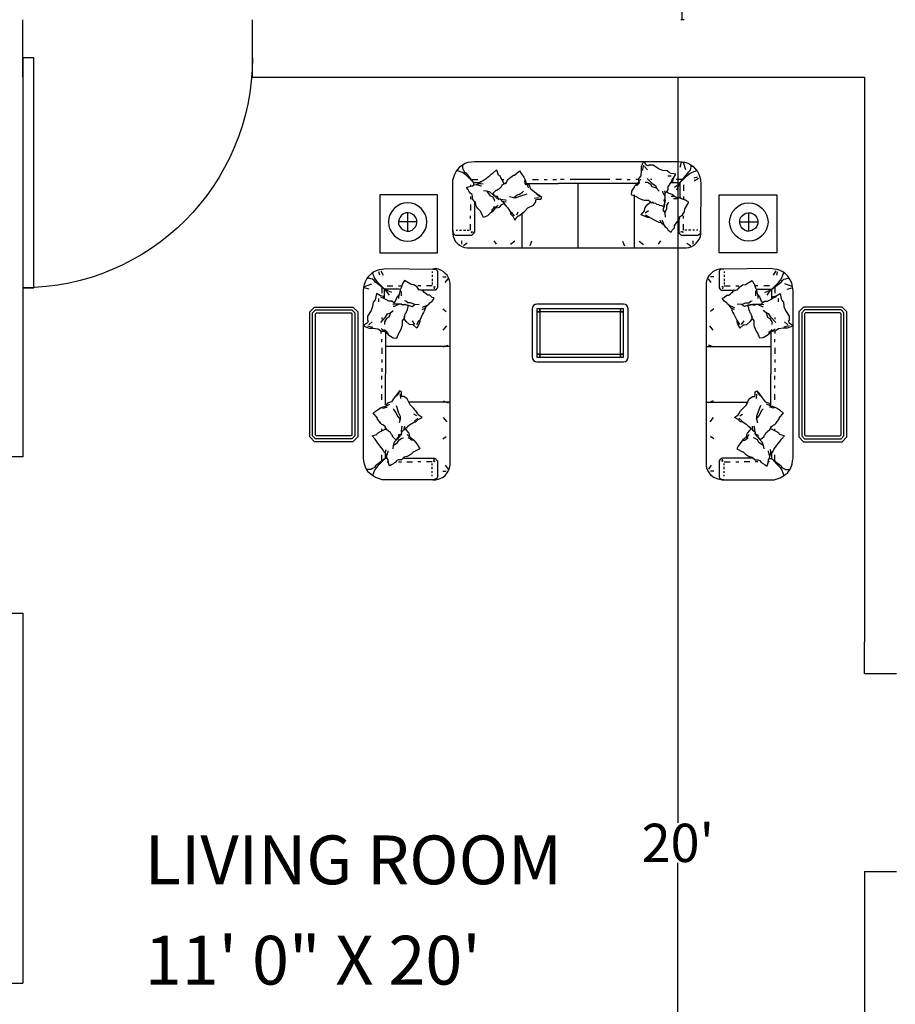
# Model space of a CAD drawing. Units: inches. Extents: x -113 to 5399, y -1393 to 3302.
# Tile 13 of 40: x 1759 to 1896, y 271 to 426. Entities that reach past the tile are written whole.
import ezdxf

# ---------------------------------------------------------------- set-up
doc = ezdxf.new("R2010")
doc.units = ezdxf.units.IN
doc.header["$MEASUREMENT"] = 0
doc.layers.add('24', color=7, linetype='Continuous')
for name, color, linetype, lineweight in [('A-ANNO-DIMS', 254, 'Continuous', 18), ('A-AREA-IDEN', 4, 'Continuous', 18), ('doors', 2, 'Continuous', 25), ('furniture', 131, 'Continuous', 18), ('walls', 1, 'Continuous', 25)]:
    doc.layers.add(name, color=color, linetype=linetype, lineweight=lineweight)
doc.styles.get("Standard").update_dxf_attribs({"font": 'arial.ttf'})
doc.dimstyles.get("Standard").update_dxf_attribs({"dimtxt": 6, "dimasz": 0.18, "dimexe": 0.18, "dimexo": 0.0625, "dimgap": 0.09, "dimtad": 0, "dimtih": 1, "dimtoh": 1, "dimdec": 1, "dimzin": 0, "dimdsep": 46, "dimlunit": 4, "dimtxsty": 'Standard', "dimblk": 'ARCHTICK', "dimcen": 0.09, "dimadec": 0, "dimazin": 0, "dimtfac": 1, "dimtdec": 1, "dimtofl": 0, "dimtmove": 0, "dimatfit": 3, "dimfxl": 1, "dimtolj": 1, "dimtzin": 0, "dimarcsym": 0})

# ---------------------------------------------------------------- blocks, each defined once
blk = doc.blocks.new('*U3')
for p, q in [((0, 0), (0, -6)), ((36, 0), (36, -6))]:
    blk.add_line(p, q)
blk.add_lwpolyline([(0, 0), (0, 36), (1.75, 36), (1.75, 0)], close=True)
blk.add_arc((0, 0), 36, 0, 90)
blk = doc.blocks.new('DL13712')
at = {"layer": '24'}
for p, q in [((33, 28.5), (-34, 28.5)), ((33.5, -29.5), (-10, -29.5))]:
    blk.add_line(p, q, dxfattribs=at)
blk = doc.blocks.new('DL13976')
at = {"layer": '24'}
for p, q in [((-18, 7.5), (-16, 11)), ((-16, 11), (-13.5, 14)), ((-13.5, 14), (-10.5, 16.5)), ((-10.5, 16.5), (-7, 18.5)), ((-7, 18.5), (-3.5, 19.5)), ((-3.5, 19.5), (0.5, 20)), ((0.5, 20), (4.5, 19.5)), ((4.5, 19.5), (8, 18.5)), ((8, 18.5), (11.5, 16.5)), ((11.5, 16.5), (14.5, 14)), ((14.5, 14), (17, 11)), ((17, 11), (19, 7.5)), ((-19.5, 0), (-19, 4)), ((-19, -4), (-19.5, 0)), ((-19, 4), (-18, 7.5)), ((-9, 2), (-8, 4.5)), ((-9, -0.5), (-9, 2)), ((-9, 0), (10, 0)), ((-8, 4.5), (-6.5, 6.5)), ((-6.5, 6.5), (-4.5, 8)), ((-5.5, 0), (6.5, 0)), ((-4.5, 8), (-2.5, 9)), ((-2.5, 9), (0, 9.5)), ((0, 9.5), (2.5, 9.5)), ((0.5, -9.5), (0.5, 9.5)), ((0.5, -6), (0.5, 6)), ((2.5, 9.5), (5, 8.5)), ((5, 8.5), (7, 7)), ((7, 7), (8.5, 5)), ((8.5, 5), (9.5, 3)), ((9.5, 3), (10, 0.5)), ((10, 0.5), (10, -2)), ((19, 7.5), (20, 4)), ((20, 4), (20.5, 0)), ((20.5, 0), (20, -4)), ((-18, -7.5), (-19, -4)), ((-16, -11), (-18, -7.5)), ((-8.5, -3), (-9, -0.5)), ((-7.5, -5), (-8.5, -3)), ((-6, -7), (-7.5, -5)), ((-4, -8.5), (-6, -7)), ((-1.5, -9.5), (-4, -8.5)), ((1, -9.5), (-1.5, -9.5)), ((3.5, -9), (1, -9.5)), ((5.5, -8), (3.5, -9)), ((7.5, -6.5), (5.5, -8)), ((9, -4.5), (7.5, -6.5)), ((10, -2), (9, -4.5)), ((19, -7.5), (17, -11)), ((20, -4), (19, -7.5)), ((-13.5, -14), (-16, -11)), ((-10.5, -16.5), (-13.5, -14)), ((-7, -18.5), (-10.5, -16.5)), ((-3.5, -19.5), (-7, -18.5)), ((0.5, -20), (-3.5, -19.5)), ((4.5, -19.5), (0.5, -20)), ((8, -18.5), (4.5, -19.5)), ((11.5, -16.5), (8, -18.5)), ((14.5, -14), (11.5, -16.5)), ((17, -11), (14.5, -14))]:
    blk.add_line(p, q, dxfattribs=at)
blk = doc.blocks.new('DL13329')
at = {"layer": '24'}
for p, q in [((0, 0), (0, -60)), ((60, 0), (0, 0)), ((60, -60), (60, 0)), ((0, -60), (60, -60))]:
    blk.add_line(p, q, dxfattribs=at)
blk = doc.blocks.new('DL13303')
at = {"layer": '24'}
for p, q in [((-70, 20), (-65, 25)), ((-67, 19), (-64, 22)), ((-65, 25), (65, 25)), ((-64, 22), (64, 22)), ((64, 22), (67, 19)), ((65, 25), (70, 20)), ((-70, -20), (-70, 20)), ((-67, -19), (-67, 19)), ((-64, 18), (-63, 19)), ((-64, -18), (-64, 18)), ((-63, 19), (63, 19)), ((63, 19), (64, 18)), ((64, 18), (64, -18)), ((67, 19), (67, -19)), ((70, 20), (70, -20)), ((-65, -25), (-70, -20)), ((-64, -22), (-67, -19)), ((-63, -19), (-64, -18)), ((63, -19), (-63, -19)), ((64, -18), (63, -19)), ((67, -19), (64, -22)), ((70, -20), (65, -25)), ((65, -25), (-65, -25)), ((64, -22), (-64, -22))]:
    blk.add_line(p, q, dxfattribs=at)
blk = doc.blocks.new('DL12701')
at = {"layer": '24'}
for p, q in [((-102, 40), (-99.5, 42)), ((-99.5, 42), (-96.5, 43.5)), ((-99, 40), (-99, 42)), ((-96.5, 43.5), (-93.5, 44.5)), ((-93.5, 44.5), (-90, 45)), ((-90, 45), (-87, 45.5)), ((-87, 45.5), (0, 45.5)), ((0, 45.5), (87, 45.5)), ((50, 45), (48, 39.5)), ((50.5, 41.5), (49, 36)), ((51.5, 44.5), (50, 45)), ((53.5, 41.5), (51.5, 44.5)), ((55.5, 40.5), (53.5, 41.5)), ((56, 41.5), (55.5, 40.5)), ((60.5, 41.5), (56, 41.5)), ((66.5, 37.5), (60.5, 41.5)), ((87, 45.5), (90.5, 45)), ((88.5, 39.5), (90, 44.5)), ((90.5, 45), (93.5, 44.5)), ((91.5, 44.5), (94, 37)), ((93.5, 44.5), (96.5, 43.5)), ((96.5, 43.5), (99.5, 42)), ((99.5, 42), (102, 40)), ((100, 40), (99.5, 42)), ((-108.5, 29), (-107.5, 32)), ((-107.5, 32), (-106, 35)), ((-106, 35), (-104, 37.5)), ((-102.5, 35), (-105, 36)), ((-104, 37.5), (-102, 40)), ((-99.5, 34), (-102.5, 35)), ((-97, 32), (-99.5, 34)), ((-99, 38), (-99, 40)), ((-98, 36), (-99, 38)), ((-97, 34), (-98, 36)), ((-95, 33), (-97, 34)), ((-95, 30.5), (-97, 32)), ((-87.5, 23), (-95, 33)), ((-71.5, 30.5), (-69.5, 32)), ((-69.5, 32), (-67.5, 33.5)), ((-67.5, 33.5), (-64, 36.5)), ((-64, 36.5), (-62.5, 31.5)), ((-62.5, 31.5), (-61, 31)), ((-61, 31), (-59.5, 28)), ((-49, 29), (-46.5, 31)), ((-46.5, 31), (-45.5, 31)), ((-45.5, 31), (-40, 35.5)), ((-40, 35.5), (-38.5, 33)), ((-38.5, 33), (-38, 32.5)), ((-38, 32.5), (-35.5, 29)), ((48, 35.5), (47.5, 30.5)), ((48, 39.5), (48, 35.5)), ((51.5, 40), (54.5, 36.5)), ((70.5, 36), (66.5, 37.5)), ((75, 35.5), (70.5, 36)), ((77.5, 33.5), (75, 35.5)), ((79, 33), (77.5, 33.5)), ((84, 32), (79, 33)), ((81.5, 28), (84, 32)), ((88.5, 23.5), (96, 33)), ((95.5, 30.5), (98, 32.5)), ((96, 33), (97.5, 34.5)), ((97.5, 34.5), (99, 36)), ((98, 32.5), (100.5, 34)), ((99, 36), (99.5, 38)), ((99.5, 38), (100, 40)), ((100.5, 34), (103, 35)), ((102, 40), (104.5, 37.5)), ((103, 35), (106, 36)), ((104.5, 37.5), (106.5, 35)), ((106.5, 35), (108, 32)), ((108, 32), (109, 29)), ((-109.5, 26), (-108.5, 29)), ((-109.5, 22.5), (-109.5, 26)), ((-109.5, -26.5), (-109.5, 22.5)), ((-87.5, 23), (-95, 30.5)), ((-91, 21), (-91, 19.5)), ((-89.5, 26.5), (-83.5, 26.5)), ((-89, 20), (-87.5, 21)), ((-87.5, 21), (-87.5, 23)), ((-81.5, 23), (-87.5, 23)), ((-87.5, 21), (-85, 21.5)), ((-85, 21.5), (-82, 22.5)), ((-85, 21.5), (-80.5, 20)), ((-82, 22.5), (-80.5, 24.5)), ((-82, 22.5), (-80.5, 22.5)), ((-80.5, 24.5), (-78, 25.5)), ((-80.5, 24.5), (-80.5, 23.5)), ((-80.5, 22.5), (-78, 22)), ((-78, 25.5), (-76, 27)), ((-77, 25.5), (-77, 25.5)), ((-76, 27), (-71.5, 30.5)), ((-59.5, 28), (-57.5, 24.5)), ((-58.5, 19.5), (-58, 21)), ((-58, 26.5), (-56.5, 26.5)), ((-58, 21), (-54.5, 23)), ((-57.5, 24.5), (-56.5, 22)), ((-56.5, 22.5), (-54.5, 22.5)), ((-54.5, 22.5), (-52.5, 25.5)), ((-54.5, 23), (-54.5, 22.5)), ((-54, 22.5), (-54, 22.5)), ((-52.5, 25.5), (-52, 26.5)), ((-52, 26.5), (-51, 27.5)), ((-51, 27.5), (-49, 29)), ((-35.5, 29), (-34.5, 27)), ((-34.5, 27), (-35, 24.5)), ((-35, 24.5), (-34.5, 23)), ((-34.5, 27), (-33.5, 24)), ((-34.5, 23), (-34, 21)), ((-33.5, 24), (-33, 22)), ((-30, 21), (-33, 22)), ((-33, 22), (-31.5, 19.5)), ((-32, 22.5), (0.5, 22.5)), ((-29.5, 19.5), (-30, 21)), ((-26.5, 26.5), (-20.5, 26.5)), ((-14.5, 26.5), (-11.5, 26.5)), ((-5.5, 26.5), (-1.5, 26.5)), ((44, 22.5), (0.5, 22.5)), ((6.5, 26.5), (2.5, 26.5)), ((15.5, 26.5), (12.5, 26.5)), ((27.5, 26.5), (21.5, 26.5)), ((33.5, 26.5), (36.5, 26.5)), ((43.5, 22), (41.5, 20)), ((43.5, 20.5), (41.5, 20)), ((42.5, 27), (45, 27)), ((45, 23.5), (43.5, 22)), ((45, 22), (43.5, 20.5)), ((45.5, 28), (45, 27)), ((45, 27), (45, 23.5)), ((45, 23.5), (46.5, 26)), ((46.5, 23.5), (45, 22)), ((47.5, 30.5), (45.5, 28)), ((46.5, 26), (47.5, 27)), ((54.5, 23.5), (52, 23.5)), ((54, 27.5), (59.5, 22.5)), ((58, 21.5), (54.5, 23.5)), ((59, 26.5), (57.5, 26.5)), ((59.5, 19), (58, 21.5)), ((59.5, 22.5), (63, 20.5)), ((63, 20.5), (64, 17.5)), ((79, 30), (75.5, 30)), ((76, 19), (79, 24)), ((80.5, 28), (79, 24)), ((79, 24), (81, 24.5)), ((79, 23.5), (88.5, 23.5)), ((81, 24.5), (81.5, 28)), ((82.5, 18.5), (88, 22.5)), ((90.5, 26.5), (84.5, 26.5)), ((85, 16), (88, 22.5)), ((88.5, 23.5), (95.5, 30.5)), ((88.5, 8), (88.5, 23.5)), ((92, 21), (92, 15)), ((103, 28.5), (106.5, 29.5)), ((107.5, 27.5), (103, 25)), ((109, 29), (109.5, 26)), ((109.5, 26), (110, 22.5)), ((110, 22.5), (109.5, -26.5)), ((-95, 18.5), (-92, 19.5)), ((-95, 18), (-95, 18.5)), ((-94, 16.5), (-95, 18)), ((-92.5, 14), (-94, 16.5)), ((-92, 13.5), (-92.5, 14)), ((-92, 19.5), (-89, 20)), ((-91.5, 12.5), (-92, 13.5)), ((-89.5, 11), (-91.5, 12.5)), ((-89, 9), (-89.5, 11)), ((-80.5, 20), (-79.5, 20)), ((-74, 14.5), (-77.5, 15)), ((-70.5, 13.5), (-74, 14.5)), ((-74, 14.5), (-71, 10)), ((-67.5, 10.5), (-70.5, 13.5)), ((-68, 12), (-67.5, 12.5)), ((-65, 9), (-68, 12)), ((-67.5, 12.5), (-66.5, 13.5)), ((-61.5, 5.5), (-67.5, 10.5)), ((-66.5, 13.5), (-64.5, 15.5)), ((-64.5, 15.5), (-63.5, 15.5)), ((-63.5, 15.5), (-62.5, 16.5)), ((-62.5, 16.5), (-60.5, 17.5)), ((-60.5, 17.5), (-59, 19.5)), ((-59, 19.5), (-58.5, 19.5)), ((-46.5, 7.5), (-42.5, 10.5)), ((-42.5, 10.5), (-40, 11.5)), ((-40, 11.5), (-37, 13.5)), ((-32.5, 11.5), (-40, 9)), ((-37, 13.5), (-36, 14.5)), ((-31.5, 19.5), (-31, 18)), ((-28.5, 16.5), (-29.5, 19.5)), ((-24.5, 13.5), (-28.5, 16.5)), ((-21, 11), (-24.5, 13.5)), ((-19, 8.5), (-22.5, 11.5)), ((-17, 8), (-21, 11)), ((38, 14), (37.5, 11)), ((37.5, 11), (43.5, 8.5)), ((40.5, 18.5), (38, 14.5)), ((38, 14.5), (38, 14)), ((41.5, 20), (40.5, 18.5)), ((64, 17.5), (59.5, 19)), ((64, 17.5), (66.5, 14.5)), ((70.5, 13.5), (70.5, 14.5)), ((73, 8.5), (70.5, 13.5)), ((73, 13), (72.5, 15)), ((73, 12.5), (75, 14.5)), ((73, 12.5), (73, 13)), ((73, 8.5), (73, 12.5)), ((76, 12.5), (74, 14)), ((75, 14.5), (76, 16)), ((75.5, 16), (76, 16.5)), ((76, 16), (76, 19)), ((80, 11), (76, 12.5)), ((80.5, 10.5), (80, 11)), ((83, 8.5), (80.5, 10.5)), ((-91, 9), (-91, 6)), ((-91, 0.5), (-91, -5.5)), ((-89, 8.5), (-89, 9)), ((-89, 6), (-89, 8.5)), ((-86.5, 3.5), (-89, 6)), ((-87, 3.5), (-87, -26.5)), ((-86, 3.5), (-86.5, 3.5)), ((-85.5, 0.5), (-86, 3.5)), ((-85.5, 0), (-85.5, 0.5)), ((-84.5, -2), (-85.5, 0)), ((-71, 10), (-68, 8.5)), ((-68, 8.5), (-66.5, 5.5)), ((-66.5, 5.5), (-66, 4)), ((-63, 9), (-65, 9)), ((-62.5, 0), (-63.5, -1)), ((-62, 6.5), (-63, 9)), ((-60, 6), (-62, 6.5)), ((-61, -2), (-58.5, 0.5)), ((-57.5, 3.5), (-60, 6)), ((-60, 6), (-55, 5.5)), ((-58.5, 0.5), (-55.5, 2)), ((-56.5, 3.5), (-57.5, 3.5)), ((-57.5, 3.5), (-56, 1.5)), ((-54, 3), (-56.5, 3.5)), ((-56, 1.5), (-55, 0)), ((-55, 5.5), (-54, 5)), ((-55, 0), (-52.5, -2.5)), ((-46.5, 7.5), (-50.5, 8.5)), ((-43.5, 7.5), (-46.5, 7.5)), ((-40, 9), (-43.5, 7.5)), ((-31.5, -3), (-25.5, 0)), ((-25.5, 0), (-23, 3.5)), ((-20.5, 7.5), (-25, 7)), ((-23, 5.5), (-21.5, 6)), ((-23, 3.5), (-23, 5.5)), ((-21.5, 6), (-18, 6)), ((-18, 6), (-17, 8)), ((43.5, 8.5), (44, 8)), ((44, 8), (47, 6.5)), ((47, 6.5), (49.5, 5.5)), ((49.5, 5.5), (51, 5)), ((51, 5), (52.5, 5)), ((52, -2.5), (55, 1)), ((52.5, 5), (55.5, 5)), ((55, 1), (57.5, 3)), ((55.5, 5), (55.5, 5)), ((55.5, 5), (59, 2.5)), ((59, 2.5), (60, 3.5)), ((60, 3.5), (60, 2.5)), ((60, 2.5), (63, 2)), ((63, 2), (64, 1)), ((64, 1), (66, 0.5)), ((66, 0.5), (66.5, 0)), ((66.5, 0), (69, -0.5)), ((71.5, -1), (72.5, 2.5)), ((72, 5), (73, 6.5)), ((73, 5.5), (72, -1)), ((72.5, 2.5), (72, 5)), ((73, 6.5), (73, 8.5)), ((74.5, -0.5), (76, 1.5)), ((76, 1.5), (76.5, 3)), ((80.5, 9), (79, 9)), ((83, 8.5), (80.5, 9)), ((84, 6.5), (81.5, 6.5)), ((85, 8), (83, 8.5)), ((85.5, 6.5), (84, 6.5)), ((88, 7.5), (85, 8)), ((88, 7.5), (85.5, 6.5)), ((90, 6.5), (88, 7.5)), ((94, 5), (90, 6.5)), ((92, 9), (92, 6)), ((95, 4.5), (94, 5)), ((94, -3), (97.5, 3)), ((97.5, 3), (95, 4.5)), ((-83, -4), (-84.5, -2)), ((-80.5, -6.5), (-83, -4)), ((-80.5, -7), (-80.5, -6.5)), ((-77.5, -13), (-80.5, -7)), ((-70.5, -8.5), (-73.5, -11)), ((-68.5, -7), (-70.5, -8.5)), ((-68.5, -4.5), (-67, -3)), ((-66.5, -4.5), (-68.5, -7)), ((-68.5, -7), (-68.5, -4.5)), ((-67, -3), (-66, -1)), ((-65.5, -3), (-66.5, -4.5)), ((-63.5, -1), (-65.5, -3)), ((-65.5, -3), (-62.5, -2.5)), ((-62.5, -2.5), (-61, -2)), ((-54, -0.5), (-53.5, -0.5)), ((-52.5, -2.5), (-49.5, -7.5)), ((-49.5, -7.5), (-49.5, -9)), ((-49.5, -9), (-47, -11.5)), ((-45.5, -11), (-48.5, -7.5)), ((-43, -10), (-41.5, -7)), ((-41, -11), (-38, -9)), ((-38, -9), (-35, -6.5)), ((-35, -6.5), (-31.5, -3)), ((48, -10), (51.5, -6)), ((52, -12), (48, -10)), ((51.5, -5.5), (52, -2.5)), ((51.5, -6), (51.5, -5.5)), ((52, -8), (55.5, -5.5)), ((52, -10), (56.5, -12.5)), ((69, -0.5), (70.5, -1)), ((70.5, -1), (71.5, -1)), ((72, -1), (70.5, -5)), ((70.5, -5), (72.5, -8)), ((72.5, -8), (74.5, -3.5)), ((72.5, -8), (73, -12.5)), ((74.5, -3.5), (74.5, -0.5)), ((89.5, -11), (91, -10)), ((91, -10), (92, -8.5)), ((92, -8.5), (93, -7)), ((93, -7), (93.5, -4)), ((93.5, -4), (94, -3)), ((-91, -14), (-91, -11)), ((-91, -26), (-91, -20)), ((-74.5, -11.5), (-77.5, -13)), ((-73.5, -11), (-74.5, -11.5)), ((-47, -11.5), (-45, -15.5)), ((-45, -15.5), (-42, -11.5)), ((-42, -11.5), (-41, -11)), ((55, -13), (52, -12)), ((56.5, -13), (55, -13)), ((62.5, -16), (56.5, -13)), ((64.5, -17), (62.5, -16)), ((64, -16.5), (64, -16.5)), ((66.5, -18), (64.5, -17)), ((69, -18.5), (66.5, -18)), ((67.5, -15.5), (68.5, -18)), ((68.5, -18), (69, -18.5)), ((69, -18.5), (72, -21)), ((70, -16.5), (69.5, -15.5)), ((72, -21), (70, -16.5)), ((82.5, -21.5), (83.5, -20)), ((83.5, -20), (85, -18)), ((85, -17.5), (87, -16.5)), ((85, -18), (85, -17.5)), ((87, -16.5), (88, -13)), ((87.5, -12.5), (89.5, -11)), ((88, -13), (87.5, -12.5)), ((87.5, -26.5), (87.5, -14.5)), ((92, -14), (92, -11)), ((92, -26), (92, -20)), ((-109.5, -28), (-109.5, -26.5)), ((-109.5, -26.5), (-109.5, -29.5)), ((-109, -29), (-109.5, -28)), ((-109.5, -29.5), (-109, -32.5)), ((-108.5, -30), (-109, -29)), ((-108, -31), (-108.5, -30)), ((-106, -26), (-104.5, -26)), ((-102.5, -26), (-100.5, -26)), ((-98.5, -26), (-96, -26)), ((-94.5, -26), (-92.5, -26)), ((-90.5, -27.5), (-88, -28)), ((-90.5, -28), (-90, -29)), ((-89, -30.5), (-90, -31.5)), ((-88, -30), (-89, -30.5)), ((-87.5, -29), (-88, -30)), ((-87, -28), (-87.5, -29)), ((-87, -26.5), (-87, -28)), ((72, -21), (73, -22.5)), ((73, -22.5), (74.5, -23.5)), ((74.5, -23.5), (76, -26)), ((76, -26), (79, -28)), ((79, -28), (79.5, -27.5)), ((79.5, -27.5), (80, -26)), ((80, -26), (82.5, -23.5)), ((82.5, -22.5), (82.5, -21.5)), ((82.5, -23.5), (82.5, -22.5)), ((87.5, -28), (87.5, -26.5)), ((87.5, -29), (87.5, -28)), ((88, -30), (87.5, -29)), ((89, -30.5), (88, -30)), ((91.5, -27.5), (89, -28)), ((90, -31.5), (89, -30.5)), ((91.5, -28), (91, -29)), ((95.5, -26), (93.5, -26)), ((99.5, -26), (97, -26)), ((103.5, -26), (101.5, -26)), ((107, -26), (105.5, -26)), ((109, -30), (108, -31)), ((109.5, -29), (109, -30)), ((110, -29.5), (109.5, -26.5)), ((109.5, -26.5), (109.5, -28)), ((109.5, -28), (109.5, -29)), ((109.5, -32.5), (110, -29.5)), ((-109, -32.5), (-108, -35)), ((-106.5, -31.5), (-108, -31)), ((-108, -35), (-107, -37.5)), ((-107, -37.5), (-105, -39.5)), ((-105.5, -31.5), (-106.5, -31.5)), ((-104.5, -31.5), (-105.5, -31.5)), ((-105, -39.5), (-102.5, -41.5)), ((-92, -31.5), (-104.5, -31.5)), ((-100.5, -37), (-100.5, -40.5)), ((-94.5, -39.5), (-98.5, -42.5)), ((-91, -31.5), (-92, -31.5)), ((-90, -31.5), (-91, -31.5)), ((-67, -37), (-64.5, -40.5)), ((-45, -37.5), (-49.5, -41)), ((-27.5, -37.5), (-29.5, -42.5)), ((28.5, -37.5), (30.5, -42.5)), ((46, -37.5), (50.5, -41)), ((68, -37), (65.5, -40.5)), ((91, -31.5), (90, -31.5)), ((92.5, -31.5), (91, -31.5)), ((104.5, -31.5), (92.5, -31.5)), ((95.5, -39.5), (99.5, -42.5)), ((101.5, -37), (101.5, -40.5)), ((103, -41.5), (105, -39.5)), ((106, -31.5), (104.5, -31.5)), ((105, -39.5), (107, -37.5)), ((107, -31.5), (106, -31.5)), ((108, -31), (107, -31.5)), ((107, -37.5), (108.5, -35)), ((108.5, -35), (109.5, -32.5)), ((-102.5, -41.5), (-100, -43)), ((-100, -43), (-97.5, -44)), ((-97.5, -44), (-94.5, -44.5)), ((-94.5, -44.5), (0, -44.5)), ((0, -44.5), (95, -44.5)), ((95, -44.5), (97.5, -44)), ((97.5, -44), (100.5, -43)), ((100.5, -43), (103, -41.5))]:
    blk.add_line(p, q, dxfattribs=at)
blk = doc.blocks.new('DL13707')
at = {"layer": '24'}
for p, q in [((0, -33.5), (0, 33.5)), ((-58.5, -33.5), (-58.5, 21.5)), ((58.5, -33.5), (58.5, 2))]:
    blk.add_line(p, q, dxfattribs=at)
blk = doc.blocks.new('DL13651')
at = {"layer": '24'}
for p, q in [((-50.5, 25), (-50, 27)), ((-50.5, -25), (-50.5, 25)), ((-50, 27), (-49, 28.5)), ((-49, 28.5), (-47.5, 29.5)), ((-47.5, 29.5), (-45.5, 30)), ((-45.5, 30), (44.5, 30)), ((-45.5, 24.5), (-45.5, 25)), ((-45.5, 25), (-45, 25)), ((-45.5, -24.5), (-45.5, 24.5)), ((-45, 25), (44, 25)), ((-45, 22), (44, 22)), ((-42.5, 22), (-45, 22)), ((-42.5, -24.5), (-42.5, 24.5)), ((-42.5, 24.5), (-42.5, 22)), ((41.5, 22), (41.5, 24.5)), ((41.5, 24.5), (41.5, -24.5)), ((44, 22), (41.5, 22)), ((44, 25), (44.5, 25)), ((44.5, 30), (46.5, 29.5)), ((44.5, 25), (44.5, 24.5)), ((44.5, 24.5), (44.5, -24.5)), ((46.5, 29.5), (48, 28.5)), ((48, 28.5), (49, 27)), ((49, 27), (49.5, 25)), ((49.5, 25), (49.5, -25)), ((-50, -27), (-50.5, -25)), ((-49, -28.5), (-50, -27)), ((-47.5, -29.5), (-49, -28.5)), ((-45.5, -30), (-47.5, -29.5)), ((-45.5, -25), (-45.5, -24.5)), ((-45, -25), (-45.5, -25)), ((44.5, -30), (-45.5, -30)), ((44, -22), (-45, -22)), ((-45, -22), (-42.5, -22)), ((44, -25), (-45, -25)), ((-42.5, -22), (-42.5, -24.5)), ((41.5, -24.5), (41.5, -22)), ((41.5, -22), (44, -22)), ((44.5, -25), (44, -25)), ((44.5, -24.5), (44.5, -25)), ((46.5, -29.5), (44.5, -30)), ((48, -28.5), (46.5, -29.5)), ((49, -27), (48, -28.5)), ((49.5, -25), (49, -27))]:
    blk.add_line(p, q, dxfattribs=at)
blk = doc.blocks.new('DL12263')
at = {"layer": '24'}
for p, q in [((-121, 40), (-118.5, 42)), ((-118.5, 42), (-115.5, 43.5)), ((-118, 40), (-118, 42)), ((-115.5, 43.5), (-112.5, 44.5)), ((-112.5, 44.5), (-109, 45)), ((-109, 45), (-106, 45.5)), ((-106, 45.5), (-19, 45.5)), ((-19, 45.5), (106.5, 45.5)), ((69.5, 45), (67.5, 39.5)), ((70, 41.5), (68.5, 36)), ((71, 44.5), (69.5, 45)), ((73, 41.5), (71, 44.5)), ((75, 40.5), (73, 41.5)), ((75.5, 41.5), (75, 40.5)), ((80, 41.5), (75.5, 41.5)), ((86, 37.5), (80, 41.5)), ((106.5, 45.5), (110, 45)), ((108, 39.5), (109.5, 44.5)), ((110, 45), (113, 44.5)), ((111, 44.5), (113.5, 37)), ((113, 44.5), (116, 43.5)), ((116, 43.5), (119, 42)), ((119, 42), (121.5, 40)), ((119.5, 40), (119, 42)), ((-127.5, 29), (-126.5, 32)), ((-126.5, 32), (-125, 35)), ((-125, 35), (-123, 37.5)), ((-121.5, 35), (-124, 36)), ((-123, 37.5), (-121, 40)), ((-118.5, 34), (-121.5, 35)), ((-116, 32), (-118.5, 34)), ((-118, 38), (-118, 40)), ((-117, 36), (-118, 38)), ((-116, 34), (-117, 36)), ((-114, 33), (-116, 34)), ((-114, 30.5), (-116, 32)), ((-106.5, 23), (-114, 33)), ((-90.5, 30.5), (-88.5, 32)), ((-88.5, 32), (-86.5, 33.5)), ((-86.5, 33.5), (-83, 36.5)), ((-83, 36.5), (-81.5, 31.5)), ((-81.5, 31.5), (-80, 31)), ((-80, 31), (-78.5, 28)), ((-68, 29), (-65.5, 31)), ((-65.5, 31), (-64.5, 31)), ((-64.5, 31), (-59, 35.5)), ((-59, 35.5), (-57.5, 33)), ((-57.5, 33), (-57, 32.5)), ((-57, 32.5), (-54.5, 29)), ((67.5, 35.5), (67, 30.5)), ((67.5, 39.5), (67.5, 35.5)), ((71, 40), (74, 36.5)), ((90, 36), (86, 37.5)), ((94.5, 35.5), (90, 36)), ((97, 33.5), (94.5, 35.5)), ((98.5, 33), (97, 33.5)), ((103.5, 32), (98.5, 33)), ((101, 28), (103.5, 32)), ((108, 23.5), (115.5, 33)), ((115, 30.5), (117.5, 32.5)), ((115.5, 33), (117, 34.5)), ((117, 34.5), (118.5, 36)), ((117.5, 32.5), (120, 34)), ((118.5, 36), (119, 38)), ((119, 38), (119.5, 40)), ((120, 34), (122.5, 35)), ((121.5, 40), (124, 37.5)), ((122.5, 35), (125.5, 36)), ((124, 37.5), (126, 35)), ((126, 35), (127.5, 32)), ((127.5, 32), (128.5, 29)), ((-128.5, 26), (-127.5, 29)), ((-128.5, 22.5), (-128.5, 26)), ((-128.5, -26.5), (-128.5, 22.5)), ((-106.5, 23), (-114, 30.5)), ((-110, 21), (-110, 19.5)), ((-108.5, 26.5), (-102.5, 26.5)), ((-108, 20), (-106.5, 21)), ((-106.5, 21), (-106.5, 23)), ((-100.5, 23), (-106.5, 23)), ((-106.5, 21), (-104, 21.5)), ((-104, 21.5), (-101, 22.5)), ((-104, 21.5), (-99.5, 20)), ((-101, 22.5), (-99.5, 24.5)), ((-101, 22.5), (-99.5, 22.5)), ((-99.5, 24.5), (-97, 25.5)), ((-99.5, 24.5), (-99.5, 23.5)), ((-99.5, 22.5), (-97, 22)), ((-97, 25.5), (-95, 27)), ((-96, 25.5), (-96, 25.5)), ((-95, 27), (-90.5, 30.5)), ((-78.5, 28), (-76.5, 24.5)), ((-77.5, 19.5), (-77, 21)), ((-77, 26.5), (-75.5, 26.5)), ((-77, 21), (-73.5, 23)), ((-76.5, 24.5), (-75.5, 22)), ((-75.5, 22.5), (-73.5, 22.5)), ((-73.5, 22.5), (-71.5, 25.5)), ((-73.5, 23), (-73.5, 22.5)), ((-73, 22.5), (-73, 22.5)), ((-71.5, 25.5), (-71, 26.5)), ((-71, 26.5), (-70, 27.5)), ((-70, 27.5), (-68, 29)), ((-54.5, 29), (-53.5, 27)), ((-53.5, 27), (-54, 24.5)), ((-54, 24.5), (-53.5, 23)), ((-53.5, 27), (-52.5, 24)), ((-53.5, 23), (-53, 21)), ((-52.5, 24), (-52, 22)), ((-49, 21), (-52, 22)), ((-52, 22), (-50.5, 19.5)), ((-51, 22.5), (-18.5, 22.5)), ((-48.5, 19.5), (-49, 21)), ((-45.5, 26.5), (-39.5, 26.5)), ((-33.5, 26.5), (-30.5, 26.5)), ((-24.5, 26.5), (-20.5, 26.5)), ((63.5, 22.5), (-18.5, 22.5)), ((-12.5, 26.5), (-16.5, 26.5)), ((35, 26.5), (-6.5, 26.5)), ((47, 26.5), (41, 26.5)), ((53, 26.5), (56, 26.5)), ((63, 22), (61, 20)), ((63, 20.5), (61, 20)), ((62, 27), (64.5, 27)), ((64.5, 23.5), (63, 22)), ((64.5, 22), (63, 20.5)), ((65, 28), (64.5, 27)), ((64.5, 27), (64.5, 23.5)), ((64.5, 23.5), (66, 26)), ((66, 23.5), (64.5, 22)), ((67, 30.5), (65, 28)), ((66, 26), (67, 27)), ((74, 23.5), (71.5, 23.5)), ((73.5, 27.5), (79, 22.5)), ((77.5, 21.5), (74, 23.5)), ((78.5, 26.5), (77, 26.5)), ((79, 19), (77.5, 21.5)), ((79, 22.5), (82.5, 20.5)), ((82.5, 20.5), (83.5, 17.5)), ((98.5, 30), (95, 30)), ((95.5, 19), (98.5, 24)), ((100, 28), (98.5, 24)), ((98.5, 24), (100.5, 24.5)), ((98.5, 23.5), (108, 23.5)), ((100.5, 24.5), (101, 28)), ((102, 18.5), (107.5, 22.5)), ((110, 26.5), (104, 26.5)), ((104.5, 16), (107.5, 22.5)), ((108, 23.5), (115, 30.5)), ((108, 8), (108, 23.5)), ((111.5, 21), (111.5, 15)), ((122.5, 28.5), (126, 29.5)), ((127, 27.5), (122.5, 25)), ((128.5, 29), (129, 26)), ((129, 26), (129.5, 22.5)), ((129.5, 22.5), (129, -26.5)), ((-114, 18.5), (-111, 19.5)), ((-114, 18), (-114, 18.5)), ((-113, 16.5), (-114, 18)), ((-111.5, 14), (-113, 16.5)), ((-111, 13.5), (-111.5, 14)), ((-111, 19.5), (-108, 20)), ((-110.5, 12.5), (-111, 13.5)), ((-108.5, 11), (-110.5, 12.5)), ((-108, 9), (-108.5, 11)), ((-99.5, 20), (-98.5, 20)), ((-93, 14.5), (-96.5, 15)), ((-89.5, 13.5), (-93, 14.5)), ((-93, 14.5), (-90, 10)), ((-86.5, 10.5), (-89.5, 13.5)), ((-87, 12), (-86.5, 12.5)), ((-84, 9), (-87, 12)), ((-86.5, 12.5), (-85.5, 13.5)), ((-80.5, 5.5), (-86.5, 10.5)), ((-85.5, 13.5), (-83.5, 15.5)), ((-83.5, 15.5), (-82.5, 15.5)), ((-82.5, 15.5), (-81.5, 16.5)), ((-81.5, 16.5), (-79.5, 17.5)), ((-79.5, 17.5), (-78, 19.5)), ((-78, 19.5), (-77.5, 19.5)), ((-65.5, 7.5), (-61.5, 10.5)), ((-61.5, 10.5), (-59, 11.5)), ((-59, 11.5), (-56, 13.5)), ((-51.5, 11.5), (-59, 9)), ((-56, 13.5), (-55, 14.5)), ((-50.5, 19.5), (-50, 18)), ((-47.5, 16.5), (-48.5, 19.5)), ((-43.5, 13.5), (-47.5, 16.5)), ((-40, 11), (-43.5, 13.5)), ((-38, 8.5), (-41.5, 11.5)), ((-36, 8), (-40, 11)), ((57.5, 14), (57, 11)), ((57, 11), (63, 8.5)), ((60, 18.5), (57.5, 14.5)), ((57.5, 14.5), (57.5, 14)), ((61, 20), (60, 18.5)), ((83.5, 17.5), (79, 19)), ((83.5, 17.5), (86, 14.5)), ((90, 13.5), (90, 14.5)), ((92.5, 8.5), (90, 13.5)), ((92.5, 13), (92, 15)), ((92.5, 12.5), (94.5, 14.5)), ((92.5, 12.5), (92.5, 13)), ((92.5, 8.5), (92.5, 12.5)), ((95.5, 12.5), (93.5, 14)), ((94.5, 14.5), (95.5, 16)), ((95, 16), (95.5, 16.5)), ((95.5, 16), (95.5, 19)), ((99.5, 11), (95.5, 12.5)), ((100, 10.5), (99.5, 11)), ((102.5, 8.5), (100, 10.5)), ((-110, 9), (-110, 6)), ((-110, 0.5), (-110, -5.5)), ((-108, 8.5), (-108, 9)), ((-108, 6), (-108, 8.5)), ((-105.5, 3.5), (-108, 6)), ((-106, 3.5), (-106, -26.5)), ((-105, 3.5), (-105.5, 3.5)), ((-104.5, 0.5), (-105, 3.5)), ((-104.5, 0), (-104.5, 0.5)), ((-103.5, -2), (-104.5, 0)), ((-90, 10), (-87, 8.5)), ((-87, 8.5), (-85.5, 5.5)), ((-85.5, 5.5), (-85, 4)), ((-82, 9), (-84, 9)), ((-81.5, 0), (-82.5, -1)), ((-81, 6.5), (-82, 9)), ((-79, 6), (-81, 6.5)), ((-80, -2), (-77.5, 0.5)), ((-76.5, 3.5), (-79, 6)), ((-79, 6), (-74, 5.5)), ((-77.5, 0.5), (-74.5, 2)), ((-75.5, 3.5), (-76.5, 3.5)), ((-76.5, 3.5), (-75, 1.5)), ((-73, 3), (-75.5, 3.5)), ((-75, 1.5), (-74, 0)), ((-74, 5.5), (-73, 5)), ((-74, 0), (-71.5, -2.5)), ((-65.5, 7.5), (-69.5, 8.5)), ((-62.5, 7.5), (-65.5, 7.5)), ((-59, 9), (-62.5, 7.5)), ((-50.5, -3), (-44.5, 0)), ((-44.5, 0), (-42, 3.5)), ((-39.5, 7.5), (-44, 7)), ((-42, 5.5), (-40.5, 6)), ((-42, 3.5), (-42, 5.5)), ((-40.5, 6), (-37, 6)), ((-37, 6), (-36, 8)), ((63, 8.5), (63.5, 8)), ((63.5, 8), (66.5, 6.5)), ((66.5, 6.5), (69, 5.5)), ((69, 5.5), (70.5, 5)), ((70.5, 5), (72, 5)), ((71.5, -2.5), (74.5, 1)), ((72, 5), (75, 5)), ((74.5, 1), (77, 3)), ((75, 5), (75, 5)), ((75, 5), (78.5, 2.5)), ((78.5, 2.5), (79.5, 3.5)), ((79.5, 3.5), (79.5, 2.5)), ((79.5, 2.5), (82.5, 2)), ((82.5, 2), (83.5, 1)), ((83.5, 1), (85.5, 0.5)), ((85.5, 0.5), (86, 0)), ((86, 0), (88.5, -0.5)), ((91, -1), (92, 2.5)), ((91.5, 5), (92.5, 6.5)), ((92.5, 5.5), (91.5, -1)), ((92, 2.5), (91.5, 5)), ((92.5, 6.5), (92.5, 8.5)), ((94, -0.5), (95.5, 1.5)), ((95.5, 1.5), (96, 3)), ((100, 9), (98.5, 9)), ((102.5, 8.5), (100, 9)), ((103.5, 6.5), (101, 6.5)), ((104.5, 8), (102.5, 8.5)), ((105, 6.5), (103.5, 6.5)), ((107.5, 7.5), (104.5, 8)), ((107.5, 7.5), (105, 6.5)), ((109.5, 6.5), (107.5, 7.5)), ((113.5, 5), (109.5, 6.5)), ((111.5, 9), (111.5, 6)), ((114.5, 4.5), (113.5, 5)), ((113.5, -3), (117, 3)), ((117, 3), (114.5, 4.5)), ((-102, -4), (-103.5, -2)), ((-99.5, -6.5), (-102, -4)), ((-99.5, -7), (-99.5, -6.5)), ((-96.5, -13), (-99.5, -7)), ((-89.5, -8.5), (-92.5, -11)), ((-87.5, -7), (-89.5, -8.5)), ((-87.5, -4.5), (-86, -3)), ((-85.5, -4.5), (-87.5, -7)), ((-87.5, -7), (-87.5, -4.5)), ((-86, -3), (-85, -1)), ((-84.5, -3), (-85.5, -4.5)), ((-82.5, -1), (-84.5, -3)), ((-84.5, -3), (-81.5, -2.5)), ((-81.5, -2.5), (-80, -2)), ((-73, -0.5), (-72.5, -0.5)), ((-71.5, -2.5), (-68.5, -7.5)), ((-68.5, -7.5), (-68.5, -9)), ((-68.5, -9), (-66, -11.5)), ((-64.5, -11), (-67.5, -7.5)), ((-62, -10), (-60.5, -7)), ((-60, -11), (-57, -9)), ((-57, -9), (-54, -6.5)), ((-54, -6.5), (-50.5, -3)), ((67.5, -10), (71, -6)), ((71.5, -12), (67.5, -10)), ((71, -5.5), (71.5, -2.5)), ((71, -6), (71, -5.5)), ((71.5, -8), (75, -5.5)), ((71.5, -10), (76, -12.5)), ((88.5, -0.5), (90, -1)), ((90, -1), (91, -1)), ((91.5, -1), (90, -5)), ((90, -5), (92, -8)), ((92, -8), (94, -3.5)), ((92, -8), (92.5, -12.5)), ((94, -3.5), (94, -0.5)), ((109, -11), (110.5, -10)), ((110.5, -10), (111.5, -8.5)), ((111.5, -8.5), (112.5, -7)), ((112.5, -7), (113, -4)), ((113, -4), (113.5, -3)), ((-110, -14), (-110, -11)), ((-110, -26), (-110, -20)), ((-93.5, -11.5), (-96.5, -13)), ((-92.5, -11), (-93.5, -11.5)), ((-66, -11.5), (-64, -15.5)), ((-64, -15.5), (-61, -11.5)), ((-61, -11.5), (-60, -11)), ((74.5, -13), (71.5, -12)), ((76, -13), (74.5, -13)), ((82, -16), (76, -13)), ((84, -17), (82, -16)), ((83.5, -16.5), (83.5, -16.5)), ((86, -18), (84, -17)), ((88.5, -18.5), (86, -18)), ((87, -15.5), (88, -18)), ((88, -18), (88.5, -18.5)), ((88.5, -18.5), (91.5, -21)), ((89.5, -16.5), (89, -15.5)), ((91.5, -21), (89.5, -16.5)), ((102, -21.5), (103, -20)), ((103, -20), (104.5, -18)), ((104.5, -17.5), (106.5, -16.5)), ((104.5, -18), (104.5, -17.5)), ((106.5, -16.5), (107.5, -13)), ((107, -12.5), (109, -11)), ((107.5, -13), (107, -12.5)), ((107, -26.5), (107, -14.5)), ((111.5, -14), (111.5, -11)), ((111.5, -26), (111.5, -20)), ((-128.5, -28), (-128.5, -26.5)), ((-128.5, -26.5), (-128.5, -29.5)), ((-128, -29), (-128.5, -28)), ((-128.5, -29.5), (-128, -32.5)), ((-127.5, -30), (-128, -29)), ((-127, -31), (-127.5, -30)), ((-125, -26), (-123.5, -26)), ((-121.5, -26), (-119.5, -26)), ((-117.5, -26), (-115, -26)), ((-113.5, -26), (-111.5, -26)), ((-109.5, -27.5), (-107, -28)), ((-109.5, -28), (-109, -29)), ((-108, -30.5), (-109, -31.5)), ((-107, -30), (-108, -30.5)), ((-106.5, -29), (-107, -30)), ((-106, -28), (-106.5, -29)), ((-106, -26.5), (-106, -28)), ((91.5, -21), (92.5, -22.5)), ((92.5, -22.5), (94, -23.5)), ((94, -23.5), (95.5, -26)), ((95.5, -26), (98.5, -28)), ((98.5, -28), (99, -27.5)), ((99, -27.5), (99.5, -26)), ((99.5, -26), (102, -23.5)), ((102, -22.5), (102, -21.5)), ((102, -23.5), (102, -22.5)), ((107, -28), (107, -26.5)), ((107, -29), (107, -28)), ((107.5, -30), (107, -29)), ((108.5, -30.5), (107.5, -30)), ((111, -27.5), (108.5, -28)), ((109.5, -31.5), (108.5, -30.5)), ((111, -28), (110.5, -29)), ((115, -26), (113, -26)), ((119, -26), (116.5, -26)), ((123, -26), (121, -26)), ((126.5, -26), (125, -26)), ((128.5, -30), (127.5, -31)), ((129, -29), (128.5, -30)), ((129.5, -29.5), (129, -26.5)), ((129, -26.5), (129, -28)), ((129, -28), (129, -29)), ((129, -32.5), (129.5, -29.5)), ((-128, -32.5), (-127, -35)), ((-125.5, -31.5), (-127, -31)), ((-127, -35), (-126, -37.5)), ((-126, -37.5), (-124, -39.5)), ((-124.5, -31.5), (-125.5, -31.5)), ((-123.5, -31.5), (-124.5, -31.5)), ((-124, -39.5), (-121.5, -41.5)), ((-111, -31.5), (-123.5, -31.5)), ((-119.5, -37), (-119.5, -40.5)), ((-113.5, -39.5), (-117.5, -42.5)), ((-110, -31.5), (-111, -31.5)), ((-109, -31.5), (-110, -31.5)), ((-86, -37), (-83.5, -40.5)), ((-64, -37.5), (-68.5, -41)), ((-46.5, -37.5), (-48.5, -42.5)), ((48, -37.5), (50, -42.5)), ((65.5, -37.5), (70, -41)), ((87.5, -37), (85, -40.5)), ((110.5, -31.5), (109.5, -31.5)), ((112, -31.5), (110.5, -31.5)), ((124, -31.5), (112, -31.5)), ((115, -39.5), (119, -42.5)), ((121, -37), (121, -40.5)), ((122.5, -41.5), (124.5, -39.5)), ((125.5, -31.5), (124, -31.5)), ((124.5, -39.5), (126.5, -37.5)), ((126.5, -31.5), (125.5, -31.5)), ((127.5, -31), (126.5, -31.5)), ((126.5, -37.5), (128, -35)), ((128, -35), (129, -32.5)), ((-121.5, -41.5), (-119, -43)), ((-119, -43), (-116.5, -44)), ((-116.5, -44), (-113.5, -44.5)), ((-113.5, -44.5), (-19, -44.5)), ((-19, -44.5), (114.5, -44.5)), ((114.5, -44.5), (117, -44)), ((117, -44), (120, -43)), ((120, -43), (122.5, -41.5))]:
    blk.add_line(p, q, dxfattribs=at)
blk = doc.blocks.new('U3M')
at = {"yscale": 10, "zscale": 10}
for name, p, xscale, rotation in [('DL13303', (1315, 2544), -10, 180), ('DL13976', (-270, 1769), 10, 90), ('DL13712', (1310, 1664), -10, 90), ('DL12263', (-445, 20), -10, 90), ('DL13707', (-335, 0), 10, 90), ('DL13651', (885, -25), 10, 270), ('DL13712', (1310, -1664), 10, 90), ('DL12701', (1315, -1779), 10, 180), ('DL13329', (50, -2064), 10, 180), ('DL13976', (-270, -1769), -10, 90)]:
    blk.add_blockref(name, p, dxfattribs=dict(at, xscale=xscale, rotation=rotation))
for name, p, xscale in [('DL12701', (1315, 1779), -10), ('DL13329', (50, 2064), -10), ('DL13303', (1315, -2544), 10)]:
    blk.add_blockref(name, p, dxfattribs=dict(at, xscale=xscale))
at = {"flags": 3}
for tag in ['AECLAY', 'AECGTYPE']:
    blk.add_attdef(tag, (0, 0), '', height=0.5, dxfattribs=at)
blk = doc.blocks.new('_ArchTick')
at = {"color": 0, "linetype": 'ByBlock', "const_width": 0.15}
blk.add_lwpolyline([(-0.5, -0.5), (0.5, 0.5)], dxfattribs=at)
blk = doc.blocks.new('*D55')
at = {"layer": 'A-ANNO-DIMS', "color": 0, "lineweight": -2, "transparency": 16777216}
for p, q in [((1862.98, 497.53), (1862.46, 497.53)), ((1862.64, 497.53), (1862.64, 464.69)), ((1862.64, 425.53), (1862.64, 458.38)), ((1862.98, 425.53), (1862.46, 425.53))]:
    blk.add_line(p, q, dxfattribs=at)
at = {"layer": 'Defpoints', "color": 0, "transparency": 16777216}
for p in [(1863.04, 497.53), (1862.64, 425.53), (1863.04, 425.53)]:
    blk.add_point(p, dxfattribs=at)
at = {"layer": 'A-ANNO-DIMS', "color": 0, "lineweight": -2, "transparency": 16777216, "xscale": 0.18, "yscale": 0.18, "zscale": 0.18}
for p, rotation in [((1862.64, 497.53), 90), ((1862.64, 425.53), 270)]:
    blk.add_blockref('_ArchTick', p, dxfattribs=dict(at, rotation=rotation))
at = {"layer": 'A-ANNO-DIMS', "color": 0, "transparency": 16777216, "insert": (1862.64, 461.53), "char_height": 6, "attachment_point": 5}
blk.add_mtext("\\A1;6'", dxfattribs=at)
blk = doc.blocks.new('*D61')
at = {"layer": 'A-ANNO-DIMS', "color": 0, "lineweight": -2, "transparency": 16777216}
for p, q in [((1861.97, 416.53), (1861.97, 299.69)), ((1862.03, 416.53), (1862.15, 416.53)), ((1861.97, 176.53), (1861.97, 293.38)), ((1862.03, 176.53), (1862.15, 176.53))]:
    blk.add_line(p, q, dxfattribs=at)
at = {"layer": 'Defpoints', "color": 0, "transparency": 16777216}
for p in [(1861.97, 416.53), (1861.97, 416.53), (1861.97, 176.53)]:
    blk.add_point(p, dxfattribs=at)
at = {"layer": 'A-ANNO-DIMS', "color": 0, "lineweight": -2, "transparency": 16777216, "xscale": 0.18, "yscale": 0.18, "zscale": 0.18}
for p, rotation in [((1861.97, 416.53), 90), ((1861.97, 176.53), 270)]:
    blk.add_blockref('_ArchTick', p, dxfattribs=dict(at, rotation=rotation))
at = {"layer": 'A-ANNO-DIMS', "color": 0, "transparency": 16777216, "insert": (1861.97, 296.53), "char_height": 6, "attachment_point": 5}
blk.add_mtext("\\A1;20'", dxfattribs=at)
blk = doc.blocks.new('*D209')
at = {"layer": 'A-ANNO-DIMS', "color": 0, "lineweight": -2, "transparency": 16777216}
for p, q in [((1754.32, 798.03), (2074.39, 798.03)), ((2074.21, 798.03), (2074.21, 467.19)), ((2074.21, 130.03), (2074.21, 460.88)), ((1754.32, 130.03), (2074.39, 130.03))]:
    blk.add_line(p, q, dxfattribs=at)
at = {"layer": 'Defpoints', "color": 0, "transparency": 16777216}
for p in [(1754.26, 798.03), (2074.21, 798.03), (1754.26, 130.03)]:
    blk.add_point(p, dxfattribs=at)
at = {"layer": 'A-ANNO-DIMS', "color": 0, "lineweight": -2, "transparency": 16777216, "xscale": 0.18, "yscale": 0.18, "zscale": 0.18}
for p, rotation in [((2074.21, 798.03), 90), ((2074.21, 130.03), 270)]:
    blk.add_blockref('_ArchTick', p, dxfattribs=dict(at, rotation=rotation))
at = {"layer": 'A-ANNO-DIMS', "color": 0, "transparency": 16777216, "insert": (2074.21, 464.03), "char_height": 6, "attachment_point": 5}
blk.add_mtext('\\A1;55\'-8"', dxfattribs=at)

msp = doc.modelspace()

# ---------------------------------------------------------------- linework, layer by layer
at = {"layer": 'walls'}
for p, q in [((1759.26, 416.53), (1759.26, 425.53)), ((1795.26, 416.53), (1795.26, 425.53)), ((1759.26, 416.53), (1759.26, 357.03)), ((1795.26, 416.53), (1891.26, 416.53)), ((1891.26, 416.53), (1891.26, 328.03)), ((1759.26, 357.03), (1735.26, 357.03)), ((1754.26, 332.53), (1759.26, 332.53)), ((1759.26, 332.53), (1759.26, 274.53)), ((1891.26, 323.03), (1891.26, 328.03)), ((1896.26, 323.03), (1891.26, 323.03)), ((1891.26, 292.03), (1891.26, 217.53)), ((1891.26, 292.03), (1896.26, 292.03)), ((1754.26, 274.53), (1759.26, 274.53))]:
    msp.add_line(p, q, dxfattribs=at)

# ---------------------------------------------------------------- block references
at = {"layer": 'doors', "xscale": -1, "rotation": 180}
msp.add_blockref('*U3', (1759.26, 419.53), dxfattribs=at)
at = {"layer": 'furniture', "xscale": -0.0150724250692195, "yscale": 0.0150724250692195, "zscale": 0.0150724250692195, "rotation": 90}
msp.add_blockref('U3M', (1846.36, 389.77), dxfattribs=at)

# ---------------------------------------------------------------- texts
at = {"layer": 'A-AREA-IDEN'}
for s, p in [('LIVING ROOM', (1778.39, 290.04)), ('11\' 0" X 20\'', (1778.39, 274.32))]:
    msp.add_text(s, height=7.6473, dxfattribs=at).set_placement(p)

# ---------------------------------------------------------------- dimensions: what is measured, and where the dimension line sits
at = {"layer": 'A-ANNO-DIMS'}
for base, p1, p2, override, picture, middle in [((2074.21, 798.03), (1754.26, 130.03), (1754.26, 798.03), {"dimdec": 1, "dimlfac": 1, "dimrnd": 0, "dimzin": 1, "dimdsep": 46, "dimlunit": 4, "dimfrac": 2}, '*D209', (2074.21, 464.03)), ((1862.64, 425.53), (1863.04, 497.53), (1863.04, 425.53), {"dimclrd": 0, "dimclre": 0, "dimclrt": 0}, '*D55', (1862.64, 461.53)), ((1861.97, 416.53), (1861.97, 176.53), (1861.97, 416.53), {"dimclrd": 0, "dimclre": 0, "dimclrt": 0}, '*D61', (1861.97, 296.53))]:
    dim = msp.add_linear_dim(base=base, p1=p1, p2=p2, angle=90, dimstyle='Standard', override=override, dxfattribs=at)
    dim.commit()
    dim.dimension.update_dxf_attribs({"geometry": picture, "text_midpoint": middle})

doc.saveas('drawing.dxf')
